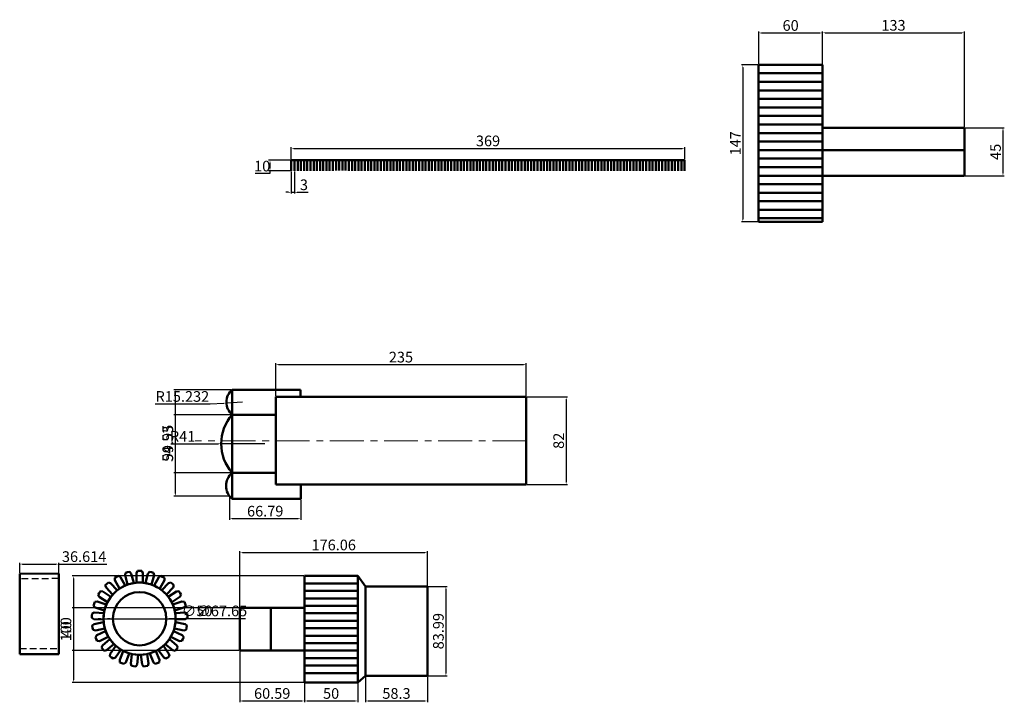
# Model space of a CAD drawing. Units: millimetres. Extents: x 828 to 2987, y 979 to 1807.
# Tile 6 of 6: x 2063 to 2987, y 979 to 1619. Entities that reach past the tile are written whole.
import ezdxf

# ---------------------------------------------------------------- set-up
doc = ezdxf.new("R2010")
doc.units = ezdxf.units.MM
doc.linetypes.add('CENTER', pattern=[50.8, 31.75, -6.35, 6.35, -6.35])
doc.linetypes.add('HIDDEN', pattern=[9.525, 6.35, -3.175])
for name, color, linetype, lineweight in [('M-CNTR', 1, 'CENTER', 18), ('M-DIMS', 2, 'Continuous', 25), ('M-HIDN', 4, 'HIDDEN', 25), ('M-OUTL', 7, 'Continuous', 50)]:
    doc.layers.add(name, color=color, linetype=linetype, lineweight=lineweight)
doc.styles.get("Standard").update_dxf_attribs({"font": 'arial.ttf'})
doc.dimstyles.new('ISO-25', dxfattribs={"dimtxt": 10, "dimasz": 2.5, "dimexe": 1.25, "dimexo": 0.625, "dimtad": 1, "dimtoh": 1, "dimdec": 0, "dimtxsty": 'Standard', "dimcen": 2.5, "dimadec": 0, "dimazin": 0, "dimtfac": 1, "dimtdec": 0, "dimtmove": 0, "dimatfit": 3, "dimfxl": 1, "dimarcsym": 0})

# ---------------------------------------------------------------- blocks, each defined once
blk = doc.blocks.new('*U61')
for p, q in [((-2, 5.46), (-3, 3.44)), ((-3, -5.56), (-3, 3.44)), ((0, 5.56), (-2, 5.46)), ((0, 5.56), (2, 5.46)), ((2, 5.46), (3, 3.44)), ((3, -5.56), (3, 3.44)), ((0, -5.56), (-3, -5.56)), ((0, -5.56), (3, -5.56))]:
    blk.add_line(p, q)
blk = doc.blocks.new('*U62')
at = {"layer": 'M-OUTL', "color": 0, "linetype": 'ByBlock', "lineweight": -2, "transparency": 16777216}
for p, rotation in [((2165.96, 1095.24), 14.39999999999996), ((2185.55, 1095.24), 345.6), ((2148.79, 1085.8), 43.20000000000002), ((2156.78, 1091.6), 28.79999999999999), ((2194.73, 1091.6), 331.2), ((2202.71, 1085.8), 316.8), ((2142.5, 1078.2), 57.6), ((2209.01, 1078.2), 302.4000000000001), ((2138.3, 1069.26), 72), ((2213.21, 1069.26), 288), ((2136.45, 1059.57), 86.40000000000002), ((2215.06, 1059.57), 273.6), ((2137.07, 1049.71), 100.8), ((2214.44, 1049.71), 259.2), ((2140.12, 1040.32), 115.2), ((2211.39, 1040.32), 244.7999999999999), ((2145.41, 1031.99), 129.6), ((2206.1, 1031.99), 230.4), ((2152.6, 1025.23), 144), ((2161.25, 1020.47), 158.4), ((2190.25, 1020.47), 201.6), ((2198.9, 1025.23), 216), ((2170.82, 1018.02), 172.8000000000001), ((2180.69, 1018.02), 187.1999999999999)]:
    blk.add_blockref('*U61', p, dxfattribs=dict(at, rotation=rotation))
blk.add_blockref('*U61', (2175.75, 1096.48), dxfattribs=at)
blk = doc.blocks.new('*D63')
at = {"layer": 'Defpoints', "color": 0, "transparency": 16777216}
for p in [(2538.55, 1265.06), (2538.55, 1182.82), (2576.02, 1182.82)]:
    blk.add_point(p, dxfattribs=at)
at = {"layer": 'M-DIMS', "color": 0, "lineweight": -2, "transparency": 16777216}
for p, q in [((2539.18, 1265.06), (2577.27, 1265.06)), ((2576.02, 1262.56), (2576.02, 1185.32)), ((2539.18, 1182.82), (2577.27, 1182.82))]:
    blk.add_line(p, q, dxfattribs=at)
at = {"layer": 'M-DIMS', "color": 0, "transparency": 16777216}
for points in [[(2575.61, 1262.56), (2576.44, 1262.56), (2576.02, 1265.06)], [(2575.61, 1185.32), (2576.44, 1185.32), (2576.02, 1182.82)]]:
    blk.add_solid(points, dxfattribs=at)
at = {"layer": 'M-DIMS', "color": 0, "transparency": 16777216, "insert": (2570.29, 1223.94), "char_height": 10, "attachment_point": 5, "rotation": 90}
blk.add_mtext('82', dxfattribs=at)
blk = doc.blocks.new('*D64')
at = {"layer": 'Defpoints', "color": 0, "transparency": 16777216}
for p in [(2538.55, 1295.39), (2303.51, 1265.06), (2538.55, 1265.06)]:
    blk.add_point(p, dxfattribs=at)
at = {"layer": 'M-DIMS', "color": 0, "lineweight": -2, "transparency": 16777216}
for p, q in [((2303.51, 1265.68), (2303.51, 1296.64)), ((2306.01, 1295.39), (2536.05, 1295.39)), ((2538.55, 1265.68), (2538.55, 1296.64))]:
    blk.add_line(p, q, dxfattribs=at)
at = {"layer": 'M-DIMS', "color": 0, "transparency": 16777216}
for points in [[(2306.01, 1295.8), (2306.01, 1294.97), (2303.51, 1295.39)], [(2536.05, 1295.8), (2536.05, 1294.97), (2538.55, 1295.39)]]:
    blk.add_solid(points, dxfattribs=at)
at = {"layer": 'M-DIMS', "color": 0, "transparency": 16777216, "insert": (2421.03, 1301.12), "char_height": 10, "attachment_point": 5}
blk.add_mtext('235', dxfattribs=at)
blk = doc.blocks.new('*D65')
at = {"layer": 'Defpoints', "color": 0, "transparency": 16777216}
for p in [(2687.32, 1498.16), (2318.12, 1487.03), (2687.32, 1487.03)]:
    blk.add_point(p, dxfattribs=at)
at = {"layer": 'M-DIMS', "color": 0, "lineweight": -2, "transparency": 16777216}
for p, q in [((2318.12, 1487.66), (2318.12, 1499.41)), ((2320.62, 1498.16), (2684.82, 1498.16)), ((2687.32, 1487.66), (2687.32, 1499.41))]:
    blk.add_line(p, q, dxfattribs=at)
at = {"layer": 'M-DIMS', "color": 0, "transparency": 16777216}
for points in [[(2320.62, 1498.57), (2320.62, 1497.74), (2318.12, 1498.16)], [(2684.82, 1498.57), (2684.82, 1497.74), (2687.32, 1498.16)]]:
    blk.add_solid(points, dxfattribs=at)
at = {"layer": 'M-DIMS', "color": 0, "transparency": 16777216, "insert": (2502.72, 1503.89), "char_height": 10, "attachment_point": 5}
blk.add_mtext('369', dxfattribs=at)
blk = doc.blocks.new('*D66')
at = {"layer": 'Defpoints', "color": 0, "transparency": 16777216}
for p in [(2816.67, 1606.42), (2756.67, 1576.58), (2816.67, 1576.58)]:
    blk.add_point(p, dxfattribs=at)
at = {"layer": 'M-DIMS', "color": 0, "lineweight": -2, "transparency": 16777216}
for p, q in [((2756.67, 1577.2), (2756.67, 1607.67)), ((2816.67, 1577.2), (2816.67, 1607.67)), ((2759.17, 1606.42), (2814.17, 1606.42))]:
    blk.add_line(p, q, dxfattribs=at)
at = {"layer": 'M-DIMS', "color": 0, "transparency": 16777216}
for points in [[(2759.17, 1606.84), (2759.17, 1606.01), (2756.67, 1606.42)], [(2814.17, 1606.84), (2814.17, 1606.01), (2816.67, 1606.42)]]:
    blk.add_solid(points, dxfattribs=at)
at = {"layer": 'M-DIMS', "color": 0, "transparency": 16777216, "insert": (2786.67, 1612.15), "char_height": 10, "attachment_point": 5}
blk.add_mtext('60', dxfattribs=at)
blk = doc.blocks.new('*D67')
at = {"layer": 'Defpoints', "color": 0, "transparency": 16777216}
for p in [(2756.67, 1576.58), (2741.8, 1429.28), (2756.67, 1429.28)]:
    blk.add_point(p, dxfattribs=at)
at = {"layer": 'M-DIMS', "color": 0, "lineweight": -2, "transparency": 16777216}
for p, q in [((2756.04, 1576.58), (2740.55, 1576.58)), ((2741.8, 1574.08), (2741.8, 1431.78)), ((2756.04, 1429.28), (2740.55, 1429.28))]:
    blk.add_line(p, q, dxfattribs=at)
at = {"layer": 'M-DIMS', "color": 0, "transparency": 16777216}
for points in [[(2741.38, 1574.08), (2742.21, 1574.08), (2741.8, 1576.58)], [(2741.38, 1431.78), (2742.21, 1431.78), (2741.8, 1429.28)]]:
    blk.add_solid(points, dxfattribs=at)
at = {"layer": 'M-DIMS', "color": 0, "transparency": 16777216, "insert": (2736.15, 1502.93), "char_height": 10, "attachment_point": 5, "rotation": 90}
blk.add_mtext('147', dxfattribs=at)
blk = doc.blocks.new('*D68')
at = {"layer": 'Defpoints', "color": 0, "transparency": 16777216}
for p in [(2949.69, 1606.56), (2816.67, 1517.31), (2949.69, 1517.31)]:
    blk.add_point(p, dxfattribs=at)
at = {"layer": 'M-DIMS', "color": 0, "lineweight": -2, "transparency": 16777216}
for p, q in [((2816.67, 1517.93), (2816.67, 1607.81)), ((2949.69, 1517.93), (2949.69, 1607.81)), ((2819.17, 1606.56), (2947.19, 1606.56))]:
    blk.add_line(p, q, dxfattribs=at)
at = {"layer": 'M-DIMS', "color": 0, "transparency": 16777216}
for points in [[(2819.17, 1606.98), (2819.17, 1606.14), (2816.67, 1606.56)], [(2947.19, 1606.98), (2947.19, 1606.14), (2949.69, 1606.56)]]:
    blk.add_solid(points, dxfattribs=at)
at = {"layer": 'M-DIMS', "color": 0, "transparency": 16777216, "insert": (2883.18, 1612.29), "char_height": 10, "attachment_point": 5}
blk.add_mtext('133', dxfattribs=at)
blk = doc.blocks.new('*D69')
at = {"layer": 'Defpoints', "color": 0, "transparency": 16777216}
for p in [(2949.69, 1517.31), (2949.69, 1472.54), (2985.91, 1472.54)]:
    blk.add_point(p, dxfattribs=at)
at = {"layer": 'M-DIMS', "color": 0, "lineweight": -2, "transparency": 16777216}
for p, q in [((2950.32, 1517.31), (2987.16, 1517.31)), ((2985.91, 1514.81), (2985.91, 1475.04)), ((2950.32, 1472.54), (2987.16, 1472.54))]:
    blk.add_line(p, q, dxfattribs=at)
at = {"layer": 'M-DIMS', "color": 0, "transparency": 16777216}
for points in [[(2985.49, 1514.81), (2986.33, 1514.81), (2985.91, 1517.31)], [(2985.49, 1475.04), (2986.33, 1475.04), (2985.91, 1472.54)]]:
    blk.add_solid(points, dxfattribs=at)
at = {"layer": 'M-DIMS', "color": 0, "transparency": 16777216, "insert": (2980.2, 1494.92), "char_height": 10, "attachment_point": 5, "rotation": 90}
blk.add_mtext('45', dxfattribs=at)
blk = doc.blocks.new('*D99')
at = {"layer": 'Defpoints', "color": 0, "transparency": 16777216}
for p in [(2318.12, 1487.03), (2298.12, 1477.03), (2318.12, 1477.03)]:
    blk.add_point(p, dxfattribs=at)
at = {"layer": 'M-DIMS', "color": 0, "lineweight": -2, "transparency": 16777216}
for p, q in [((2317.49, 1487.03), (2296.87, 1487.03)), ((2298.12, 1484.53), (2298.12, 1479.53)), ((2298.12, 1474.53), (2284.14, 1474.53)), ((2317.49, 1477.03), (2296.87, 1477.03)), ((2298.12, 1477.03), (2298.12, 1474.53))]:
    blk.add_line(p, q, dxfattribs=at)
at = {"layer": 'M-DIMS', "color": 0, "transparency": 16777216}
for points in [[(2297.7, 1484.53), (2298.53, 1484.53), (2298.12, 1487.03)], [(2297.7, 1479.53), (2298.53, 1479.53), (2298.12, 1477.03)]]:
    blk.add_solid(points, dxfattribs=at)
at = {"layer": 'M-DIMS', "color": 0, "transparency": 16777216, "insert": (2290.82, 1480.26), "char_height": 10, "attachment_point": 5}
blk.add_mtext('10', dxfattribs=at)
blk = doc.blocks.new('*D100')
at = {"layer": 'Defpoints', "color": 0, "transparency": 16777216}
for p in [(2318.12, 1477.03), (2321.12, 1477.03), (2321.12, 1456.98)]:
    blk.add_point(p, dxfattribs=at)
at = {"layer": 'M-DIMS', "color": 0, "lineweight": -2, "transparency": 16777216}
for p, q in [((2318.12, 1476.41), (2318.12, 1455.73)), ((2321.12, 1476.41), (2321.12, 1455.73)), ((2315.62, 1456.98), (2313.12, 1456.98)), ((2318.12, 1456.98), (2321.12, 1456.98)), ((2323.62, 1456.98), (2333.91, 1456.98))]:
    blk.add_line(p, q, dxfattribs=at)
at = {"layer": 'M-DIMS', "color": 0, "transparency": 16777216}
for points in [[(2315.62, 1457.4), (2315.62, 1456.57), (2318.12, 1456.98)], [(2323.62, 1457.4), (2323.62, 1456.57), (2321.12, 1456.98)]]:
    blk.add_solid(points, dxfattribs=at)
at = {"layer": 'M-DIMS', "color": 0, "transparency": 16777216, "insert": (2330.01, 1462.72), "char_height": 10, "attachment_point": 5}
blk.add_mtext('3', dxfattribs=at)
blk = doc.blocks.new('*D101')
at = {"layer": 'Defpoints', "color": 0, "transparency": 16777216}
for p in [(2262.71, 1271.88), (2209.27, 1171.93), (2260.25, 1171.93)]:
    blk.add_point(p, dxfattribs=at)
at = {"layer": 'M-DIMS', "color": 0, "lineweight": -2, "transparency": 16777216}
for p, q in [((2262.09, 1271.88), (2208.02, 1271.88)), ((2209.27, 1269.38), (2209.27, 1174.43)), ((2259.62, 1171.93), (2208.02, 1171.93))]:
    blk.add_line(p, q, dxfattribs=at)
at = {"layer": 'M-DIMS', "color": 0, "transparency": 16777216}
for points in [[(2208.85, 1269.38), (2209.68, 1269.38), (2209.27, 1271.88)], [(2208.85, 1174.43), (2209.68, 1174.43), (2209.27, 1171.93)]]:
    blk.add_solid(points, dxfattribs=at)
at = {"layer": 'M-DIMS', "color": 0, "transparency": 16777216, "insert": (2203.54, 1221.9), "char_height": 10, "attachment_point": 5, "rotation": 90}
blk.add_mtext('99.95', dxfattribs=at)
blk = doc.blocks.new('*D102')
at = {"layer": 'Defpoints', "color": 0, "transparency": 16777216}
for p in [(2262.71, 1248.42), (2209.27, 1193.89), (2262.71, 1193.89)]:
    blk.add_point(p, dxfattribs=at)
at = {"layer": 'M-DIMS', "color": 0, "lineweight": -2, "transparency": 16777216}
for p, q in [((2262.09, 1248.42), (2208.02, 1248.42)), ((2209.27, 1245.92), (2209.27, 1196.39)), ((2262.09, 1193.89), (2208.02, 1193.89))]:
    blk.add_line(p, q, dxfattribs=at)
at = {"layer": 'M-DIMS', "color": 0, "transparency": 16777216}
for points in [[(2208.85, 1245.92), (2209.68, 1245.92), (2209.27, 1248.42)], [(2208.85, 1196.39), (2209.68, 1196.39), (2209.27, 1193.89)]]:
    blk.add_solid(points, dxfattribs=at)
at = {"layer": 'M-DIMS', "color": 0, "transparency": 16777216, "insert": (2203.53, 1221.16), "char_height": 10, "attachment_point": 5, "rotation": 90}
blk.add_mtext('54.53', dxfattribs=at)
blk = doc.blocks.new('*D103')
at = {"layer": 'Defpoints', "color": 0, "transparency": 16777216}
for p in [(2260.25, 1171.93), (2327.04, 1169.42), (2327.04, 1150.92)]:
    blk.add_point(p, dxfattribs=at)
at = {"layer": 'M-DIMS', "color": 0, "lineweight": -2, "transparency": 16777216}
for p, q in [((2260.25, 1171.31), (2260.25, 1149.67)), ((2327.04, 1168.8), (2327.04, 1149.67)), ((2262.75, 1150.92), (2324.54, 1150.92))]:
    blk.add_line(p, q, dxfattribs=at)
at = {"layer": 'M-DIMS', "color": 0, "transparency": 16777216}
for points in [[(2262.75, 1151.34), (2262.75, 1150.51), (2260.25, 1150.92)], [(2324.54, 1151.34), (2324.54, 1150.51), (2327.04, 1150.92)]]:
    blk.add_solid(points, dxfattribs=at)
at = {"layer": 'M-DIMS', "color": 0, "transparency": 16777216, "insert": (2293.64, 1156.65), "char_height": 10, "attachment_point": 5}
blk.add_mtext('66.79', dxfattribs=at)
blk = doc.blocks.new('*D104')
at = {"layer": 'Defpoints', "color": 0, "transparency": 16777216}
for p in [(2099.87, 1108.29), (2063.26, 1099.09), (2099.87, 1099.39)]:
    blk.add_point(p, dxfattribs=at)
at = {"layer": 'M-DIMS', "color": 0, "lineweight": -2, "transparency": 16777216}
for p, q in [((2063.26, 1099.71), (2063.26, 1109.54)), ((2099.87, 1100.01), (2099.87, 1109.54)), ((2065.76, 1108.29), (2097.37, 1108.29)), ((2099.87, 1108.29), (2145.09, 1108.29))]:
    blk.add_line(p, q, dxfattribs=at)
at = {"layer": 'M-DIMS', "color": 0, "transparency": 16777216}
for points in [[(2065.76, 1108.7), (2065.76, 1107.87), (2063.26, 1108.29)], [(2097.37, 1108.7), (2097.37, 1107.87), (2099.87, 1108.29)]]:
    blk.add_solid(points, dxfattribs=at)
at = {"layer": 'M-DIMS', "color": 0, "transparency": 16777216, "insert": (2123.73, 1114.02), "char_height": 10, "attachment_point": 5}
blk.add_mtext('36.614', dxfattribs=at)
blk = doc.blocks.new('*D105')
at = {"layer": 'Defpoints', "color": 0, "transparency": 16777216}
for p in [(2269.9, 1027.14), (2330.49, 1027.14), (2330.49, 979.94)]:
    blk.add_point(p, dxfattribs=at)
at = {"layer": 'M-DIMS', "color": 0, "lineweight": -2, "transparency": 16777216}
for p, q in [((2269.9, 1026.51), (2269.9, 978.69)), ((2330.49, 1026.51), (2330.49, 978.69)), ((2272.4, 979.94), (2327.99, 979.94))]:
    blk.add_line(p, q, dxfattribs=at)
at = {"layer": 'M-DIMS', "color": 0, "transparency": 16777216}
for points in [[(2272.4, 980.36), (2272.4, 979.52), (2269.9, 979.94)], [(2327.99, 980.36), (2327.99, 979.52), (2330.49, 979.94)]]:
    blk.add_solid(points, dxfattribs=at)
at = {"layer": 'M-DIMS', "color": 0, "transparency": 16777216, "insert": (2300.19, 985.67), "char_height": 10, "attachment_point": 5}
blk.add_mtext('60.59', dxfattribs=at)
blk = doc.blocks.new('*D106')
at = {"layer": 'Defpoints', "color": 0, "transparency": 16777216}
for p in [(2330.49, 997.14), (2380.49, 997.14), (2380.49, 979.94)]:
    blk.add_point(p, dxfattribs=at)
at = {"layer": 'M-DIMS', "color": 0, "lineweight": -2, "transparency": 16777216}
for p, q in [((2330.49, 996.51), (2330.49, 978.69)), ((2380.49, 996.51), (2380.49, 978.69)), ((2332.99, 979.94), (2377.99, 979.94))]:
    blk.add_line(p, q, dxfattribs=at)
at = {"layer": 'M-DIMS', "color": 0, "transparency": 16777216}
for points in [[(2332.99, 980.36), (2332.99, 979.52), (2330.49, 979.94)], [(2377.99, 980.36), (2377.99, 979.52), (2380.49, 979.94)]]:
    blk.add_solid(points, dxfattribs=at)
at = {"layer": 'M-DIMS', "color": 0, "transparency": 16777216, "insert": (2355.49, 985.67), "char_height": 10, "attachment_point": 5}
blk.add_mtext('50', dxfattribs=at)
blk = doc.blocks.new('*D107')
at = {"layer": 'Defpoints', "color": 0, "transparency": 16777216}
for p in [(2387.67, 1003.41), (2445.96, 1003.41), (2445.96, 979.94)]:
    blk.add_point(p, dxfattribs=at)
at = {"layer": 'M-DIMS', "color": 0, "lineweight": -2, "transparency": 16777216}
for p, q in [((2387.67, 1002.78), (2387.67, 978.69)), ((2445.96, 1002.78), (2445.96, 978.69)), ((2390.17, 979.94), (2443.46, 979.94))]:
    blk.add_line(p, q, dxfattribs=at)
at = {"layer": 'M-DIMS', "color": 0, "transparency": 16777216}
for points in [[(2390.17, 980.36), (2390.17, 979.52), (2387.67, 979.94)], [(2443.46, 980.36), (2443.46, 979.52), (2445.96, 979.94)]]:
    blk.add_solid(points, dxfattribs=at)
at = {"layer": 'M-DIMS', "color": 0, "transparency": 16777216, "insert": (2416.82, 985.67), "char_height": 10, "attachment_point": 5}
blk.add_mtext('58.3', dxfattribs=at)
blk = doc.blocks.new('*D108')
at = {"layer": 'Defpoints', "color": 0, "transparency": 16777216}
for p in [(2445.96, 1119.23), (2269.9, 1027.14), (2445.96, 1003.41)]:
    blk.add_point(p, dxfattribs=at)
at = {"layer": 'M-DIMS', "color": 0, "lineweight": -2, "transparency": 16777216}
for p, q in [((2269.9, 1027.76), (2269.9, 1120.48)), ((2272.4, 1119.23), (2443.46, 1119.23)), ((2445.96, 1004.03), (2445.96, 1120.48))]:
    blk.add_line(p, q, dxfattribs=at)
at = {"layer": 'M-DIMS', "color": 0, "transparency": 16777216}
for points in [[(2272.4, 1119.65), (2272.4, 1118.82), (2269.9, 1119.23)], [(2443.46, 1119.65), (2443.46, 1118.82), (2445.96, 1119.23)]]:
    blk.add_solid(points, dxfattribs=at)
at = {"layer": 'M-DIMS', "color": 0, "transparency": 16777216, "insert": (2357.93, 1124.96), "char_height": 10, "attachment_point": 5}
blk.add_mtext('176.06', dxfattribs=at)
blk = doc.blocks.new('*D109')
at = {"layer": 'Defpoints', "color": 0, "transparency": 16777216}
for p in [(2269.9, 1067.14), (2113.67, 1027.14), (2269.9, 1027.14)]:
    blk.add_point(p, dxfattribs=at)
at = {"layer": 'M-DIMS', "color": 0, "lineweight": -2, "transparency": 16777216}
for p, q in [((2269.28, 1067.14), (2112.42, 1067.14)), ((2113.67, 1064.64), (2113.67, 1029.64)), ((2269.28, 1027.14), (2112.42, 1027.14))]:
    blk.add_line(p, q, dxfattribs=at)
at = {"layer": 'M-DIMS', "color": 0, "transparency": 16777216}
for points in [[(2113.25, 1064.64), (2114.09, 1064.64), (2113.67, 1067.14)], [(2113.25, 1029.64), (2114.09, 1029.64), (2113.67, 1027.14)]]:
    blk.add_solid(points, dxfattribs=at)
at = {"layer": 'M-DIMS', "color": 0, "transparency": 16777216, "insert": (2107.94, 1047.14), "char_height": 10, "attachment_point": 5, "rotation": 90}
blk.add_mtext('40', dxfattribs=at)
blk = doc.blocks.new('*D110')
at = {"layer": 'Defpoints', "color": 0, "transparency": 16777216}
for p in [(2330.49, 1097.14), (2113.67, 997.14), (2330.49, 997.14)]:
    blk.add_point(p, dxfattribs=at)
at = {"layer": 'M-DIMS', "color": 0, "lineweight": -2, "transparency": 16777216}
for p, q in [((2329.86, 1097.14), (2112.42, 1097.14)), ((2113.67, 1094.64), (2113.67, 999.64)), ((2329.86, 997.14), (2112.42, 997.14))]:
    blk.add_line(p, q, dxfattribs=at)
at = {"layer": 'M-DIMS', "color": 0, "transparency": 16777216}
for points in [[(2113.25, 1094.64), (2114.09, 1094.64), (2113.67, 1097.14)], [(2113.25, 999.64), (2114.09, 999.64), (2113.67, 997.14)]]:
    blk.add_solid(points, dxfattribs=at)
at = {"layer": 'M-DIMS', "color": 0, "transparency": 16777216, "insert": (2107.94, 1047.14), "char_height": 10, "attachment_point": 5, "rotation": 90}
blk.add_mtext('100', dxfattribs=at)
blk = doc.blocks.new('*D111')
at = {"layer": 'Defpoints', "color": 0, "transparency": 16777216}
for p in [(2445.96, 1087.4), (2445.96, 1003.41), (2463.16, 1003.41)]:
    blk.add_point(p, dxfattribs=at)
at = {"layer": 'M-DIMS', "color": 0, "lineweight": -2, "transparency": 16777216}
for p, q in [((2446.59, 1087.4), (2464.41, 1087.4)), ((2463.16, 1084.9), (2463.16, 1005.91)), ((2446.59, 1003.41), (2464.41, 1003.41))]:
    blk.add_line(p, q, dxfattribs=at)
at = {"layer": 'M-DIMS', "color": 0, "transparency": 16777216}
for points in [[(2462.75, 1084.9), (2463.58, 1084.9), (2463.16, 1087.4)], [(2462.75, 1005.91), (2463.58, 1005.91), (2463.16, 1003.41)]]:
    blk.add_solid(points, dxfattribs=at)
at = {"layer": 'M-DIMS', "color": 0, "transparency": 16777216, "insert": (2457.43, 1045.4), "char_height": 10, "attachment_point": 5, "rotation": 90}
blk.add_mtext('83.99', dxfattribs=at)
blk = doc.blocks.new('*D141')
at = {"layer": 'Defpoints', "color": 0, "transparency": 16777216}
for p in [(2252.33, 1221.16), (2293.33, 1221.16)]:
    blk.add_point(p, dxfattribs=at)
at = {"layer": 'M-DIMS', "color": 0, "lineweight": -2, "transparency": 16777216}
for p, q in [((2205.14, 1221.16), (2227.73, 1221.16)), ((2227.73, 1221.16), (2249.83, 1221.16)), ((2293.33, 1221.16), (2252.33, 1221.16))]:
    blk.add_line(p, q, dxfattribs=at)
at = {"layer": 'M-DIMS', "color": 0, "transparency": 16777216}
blk.add_solid([(2249.83, 1221.57), (2249.83, 1220.74), (2252.33, 1221.16)], dxfattribs=at)
at = {"layer": 'M-DIMS', "color": 0, "transparency": 16777216, "insert": (2216.13, 1226.8), "char_height": 10, "attachment_point": 5}
blk.add_mtext('R41', dxfattribs=at)
blk = doc.blocks.new('*D142')
at = {"layer": 'Defpoints', "color": 0, "transparency": 16777216}
for p in [(2257.22, 1259.32), (2272.43, 1260.15)]:
    blk.add_point(p, dxfattribs=at)
at = {"layer": 'M-DIMS', "color": 0, "lineweight": -2, "transparency": 16777216}
for p, q in [((2190.42, 1258.49), (2242.02, 1258.49)), ((2242.02, 1258.49), (2254.72, 1259.18)), ((2272.43, 1260.15), (2257.22, 1259.32))]:
    blk.add_line(p, q, dxfattribs=at)
at = {"layer": 'M-DIMS', "color": 0, "transparency": 16777216}
blk.add_solid([(2254.7, 1259.6), (2254.75, 1258.77), (2257.22, 1259.32)], dxfattribs=at)
at = {"layer": 'M-DIMS', "color": 0, "transparency": 16777216, "insert": (2215.91, 1264.22), "char_height": 10, "attachment_point": 5}
blk.add_mtext('R15.232', dxfattribs=at)
blk = doc.blocks.new('*D143')
at = {"layer": 'Defpoints', "color": 0, "transparency": 16777216}
for p in [(2150.75, 1057.09), (2200.75, 1057.09)]:
    blk.add_point(p, dxfattribs=at)
at = {"layer": 'M-DIMS', "color": 0, "lineweight": -2, "transparency": 16777216}
for p, q in [((2148.25, 1057.09), (2145.75, 1057.09)), ((2150.75, 1057.09), (2200.75, 1057.09)), ((2216.52, 1057.09), (2203.25, 1057.09)), ((2242.32, 1057.09), (2216.52, 1057.09))]:
    blk.add_line(p, q, dxfattribs=at)
at = {"layer": 'M-DIMS', "color": 0, "transparency": 16777216}
for points in [[(2148.25, 1057.51), (2148.25, 1056.68), (2150.75, 1057.09)], [(2203.25, 1057.51), (2203.25, 1056.68), (2200.75, 1057.09)]]:
    blk.add_solid(points, dxfattribs=at)
at = {"layer": 'M-DIMS', "color": 0, "transparency": 16777216, "insert": (2229.73, 1063.1), "char_height": 10, "attachment_point": 5}
blk.add_mtext('∅50', dxfattribs=at)
blk = doc.blocks.new('*D144')
at = {"layer": 'Defpoints', "color": 0, "transparency": 16777216}
for p in [(2141.93, 1057.09), (2209.58, 1057.09)]:
    blk.add_point(p, dxfattribs=at)
at = {"layer": 'M-DIMS', "color": 0, "lineweight": -2, "transparency": 16777216}
for p, q in [((2139.43, 1057.09), (2136.93, 1057.09)), ((2141.93, 1057.09), (2209.58, 1057.09)), ((2229.88, 1057.09), (2212.08, 1057.09)), ((2275.2, 1057.09), (2229.88, 1057.09))]:
    blk.add_line(p, q, dxfattribs=at)
at = {"layer": 'M-DIMS', "color": 0, "transparency": 16777216}
for points in [[(2139.43, 1057.51), (2139.43, 1056.68), (2141.93, 1057.09)], [(2212.08, 1057.51), (2212.08, 1056.68), (2209.58, 1057.09)]]:
    blk.add_solid(points, dxfattribs=at)
at = {"layer": 'M-DIMS', "color": 0, "transparency": 16777216, "insert": (2252.85, 1063.1), "char_height": 10, "attachment_point": 5}
blk.add_mtext('∅67.65', dxfattribs=at)

msp = doc.modelspace()

# ---------------------------------------------------------------- linework, layer by layer
at = {"layer": 'M-CNTR'}
msp.add_line((2538.5542, 1223.9389), (2227.7676, 1223.9389), dxfattribs=at)
at = {"layer": 'M-HIDN'}
for p, q in [((2099.9133, 1094.7014), (2063.2995, 1094.4015)), ((2063.2612, 1029.0021), (2099.8749, 1029.0021))]:
    msp.add_line(p, q, dxfattribs=at)
at = {"layer": 'M-OUTL'}
for p, q in [((2756.6676, 1576.5779), (2756.6676, 1429.2768)), ((2756.6676, 1576.5779), (2816.6676, 1576.5779)), ((2756.6676, 1576.5779), (2756.6676, 1568.5779)), ((2816.6676, 1429.2768), (2816.6676, 1576.5779)), ((2756.6676, 1568.5779), (2816.6676, 1568.5779)), ((2816.6676, 1560.5779), (2756.6676, 1560.5779)), ((2756.6676, 1552.5779), (2816.6676, 1552.5779)), ((2816.6676, 1544.5779), (2756.6676, 1544.5779)), ((2756.6676, 1536.5779), (2816.6676, 1536.5779)), ((2816.6676, 1528.5779), (2756.6676, 1528.5779)), ((2756.6676, 1520.5779), (2816.6676, 1520.5779)), ((2816.6676, 1517.308), (2949.693, 1517.308)), ((2949.693, 1517.308), (2949.693, 1472.5387)), ((2816.6676, 1512.5779), (2756.6676, 1512.5779)), ((2756.6676, 1504.5779), (2816.6676, 1504.5779)), ((2816.6676, 1496.5779), (2756.6676, 1496.5779)), ((2756.6676, 1488.5779), (2816.6676, 1488.5779)), ((2816.6676, 1496.5779), (2949.693, 1496.5779)), ((2318.1154, 1487.0339), (2687.1154, 1487.0339)), ((2318.1154, 1487.0339), (2318.1154, 1477.0339)), ((2321.1154, 1477.0339), (2321.1154, 1487.0339)), ((2321.1154, 1487.0339), (2324.1154, 1487.0339)), ((2324.1154, 1487.0339), (2324.1154, 1477.0339)), ((2327.1154, 1477.0339), (2327.1154, 1487.0339)), ((2330.1154, 1487.0339), (2330.1154, 1476.9825)), ((2333.1154, 1476.9825), (2333.1154, 1487.0339)), ((2336.1154, 1487.0339), (2336.1154, 1477.0762)), ((2339.1154, 1477.0762), (2339.1154, 1487.0339)), ((2342.1154, 1487.0339), (2342.1154, 1477.0339)), ((2345.1154, 1477.0339), (2345.1154, 1487.0339)), ((2348.1154, 1487.0339), (2348.1154, 1477.1476)), ((2351.1154, 1477.1476), (2351.1154, 1487.0339)), ((2354.1154, 1487.0339), (2354.1154, 1477.1238)), ((2357.1154, 1477.1238), (2357.1154, 1487.0339)), ((2360.1154, 1487.0339), (2360.1154, 1477.4097)), ((2363.1154, 1477.4097), (2363.1154, 1487.0339)), ((2366.1154, 1487.0339), (2366.1154, 1477.2911)), ((2369.1154, 1477.2911), (2369.1154, 1487.0339)), ((2372.1154, 1487.0339), (2372.1154, 1477.1482)), ((2375.1154, 1477.1482), (2375.1154, 1487.0339)), ((2378.1154, 1487.0339), (2378.1154, 1477.0474)), ((2381.1154, 1477.0474), (2381.1154, 1487.0339)), ((2384.1154, 1487.0339), (2384.1154, 1477.0857)), ((2387.1154, 1477.0857), (2387.1154, 1487.0339)), ((2390.1154, 1487.0339), (2390.1154, 1477.0339)), ((2393.1154, 1477.0339), (2393.1154, 1487.0339)), ((2396.1154, 1487.0339), (2396.1154, 1477.0339)), ((2399.1154, 1477.0339), (2399.1154, 1487.0339)), ((2402.1154, 1487.0339), (2402.1154, 1477.0339)), ((2405.1154, 1477.0339), (2405.1154, 1487.0339)), ((2408.1154, 1487.0339), (2408.1154, 1477.0339)), ((2411.1154, 1477.0339), (2411.1154, 1487.0339)), ((2414.1154, 1487.0339), (2414.1154, 1477.0339)), ((2417.1154, 1477.0339), (2417.1154, 1487.0339)), ((2420.1154, 1487.0339), (2420.1154, 1477.0339)), ((2423.1154, 1477.0339), (2423.1154, 1487.0339)), ((2426.1154, 1487.0339), (2426.1154, 1477.0339)), ((2429.1154, 1477.0339), (2429.1154, 1487.0339)), ((2432.1154, 1487.0339), (2432.1154, 1477.0339)), ((2435.1154, 1477.0339), (2435.1154, 1487.0339)), ((2438.1154, 1487.0339), (2438.1154, 1477.0339)), ((2441.1154, 1477.0339), (2441.1154, 1487.0339)), ((2444.1154, 1487.0339), (2444.1154, 1477.0339)), ((2447.1154, 1477.0339), (2447.1154, 1487.0339)), ((2450.1154, 1487.0339), (2450.1154, 1477.0339)), ((2453.1154, 1477.0339), (2453.1154, 1487.0339)), ((2456.1154, 1487.0339), (2456.1154, 1477.0339)), ((2459.1154, 1477.0339), (2459.1154, 1487.0339)), ((2462.1154, 1487.0339), (2462.1154, 1477.0339)), ((2465.1154, 1477.0339), (2465.1154, 1487.0339)), ((2468.1154, 1487.0339), (2468.1154, 1477.0339)), ((2471.1154, 1477.0339), (2471.1154, 1487.0339)), ((2474.1154, 1487.0339), (2474.1154, 1477.0339)), ((2477.1154, 1477.0339), (2477.1154, 1487.0339)), ((2480.1154, 1487.0339), (2480.1154, 1477.0339)), ((2483.1154, 1477.0339), (2483.1154, 1487.0339)), ((2486.1154, 1487.0339), (2486.1154, 1477.0339)), ((2489.1154, 1477.0339), (2489.1154, 1487.0339)), ((2492.1154, 1487.0339), (2492.1154, 1477.0339)), ((2495.1154, 1477.0339), (2495.1154, 1487.0339)), ((2498.1154, 1487.0339), (2498.1154, 1477.0339)), ((2501.1154, 1477.0339), (2501.1154, 1487.0339)), ((2504.1154, 1487.0339), (2504.1154, 1477.0339)), ((2507.1154, 1477.0339), (2507.1154, 1487.0339)), ((2510.1154, 1487.0339), (2510.1154, 1477.0339)), ((2513.1154, 1477.0339), (2513.1154, 1487.0339)), ((2516.1154, 1487.0339), (2516.1154, 1477.0339)), ((2519.1154, 1477.0339), (2519.1154, 1487.0339)), ((2522.1154, 1487.0339), (2522.1154, 1477.0339)), ((2525.1154, 1477.0339), (2525.1154, 1487.0339)), ((2528.1154, 1487.0339), (2528.1154, 1477.0339)), ((2531.1154, 1477.0339), (2531.1154, 1487.0339)), ((2534.1154, 1487.0339), (2534.1154, 1477.0339)), ((2537.1154, 1477.0339), (2537.1154, 1487.0339)), ((2540.1154, 1487.0339), (2540.1154, 1477.0339)), ((2543.1154, 1477.0339), (2543.1154, 1487.0339)), ((2546.1154, 1487.0339), (2546.1154, 1477.0339)), ((2549.1154, 1477.0339), (2549.1154, 1487.0339)), ((2552.1154, 1487.0339), (2552.1154, 1477.0339)), ((2555.1154, 1477.0339), (2555.1154, 1487.0339)), ((2558.1154, 1487.0339), (2558.1154, 1477.0339)), ((2561.1154, 1477.0339), (2561.1154, 1487.0339)), ((2564.1154, 1487.0339), (2564.1154, 1477.0339)), ((2567.1154, 1477.0339), (2567.1154, 1487.0339)), ((2570.1154, 1487.0339), (2570.1154, 1477.0339)), ((2573.1154, 1477.0339), (2573.1154, 1487.0339)), ((2576.1154, 1487.0339), (2576.1154, 1477.0339)), ((2579.1154, 1477.0339), (2579.1154, 1487.0339)), ((2582.1154, 1487.0339), (2582.1154, 1477.0339)), ((2585.1154, 1477.0339), (2585.1154, 1487.0339)), ((2588.1154, 1487.0339), (2588.1154, 1477.0339)), ((2591.1154, 1477.0339), (2591.1154, 1487.0339)), ((2594.1154, 1487.0339), (2594.1154, 1477.0339)), ((2597.1154, 1477.0339), (2597.1154, 1487.0339)), ((2600.1154, 1487.0339), (2600.1154, 1477.0339)), ((2603.1154, 1477.0339), (2603.1154, 1487.0339)), ((2606.1154, 1487.0339), (2606.1154, 1477.0339)), ((2609.1154, 1477.0339), (2609.1154, 1487.0339)), ((2612.1154, 1487.0339), (2612.1154, 1477.0339)), ((2615.1154, 1477.0339), (2615.1154, 1487.0339)), ((2618.1154, 1487.0339), (2618.1154, 1477.0339)), ((2621.1154, 1477.0339), (2621.1154, 1487.0339)), ((2624.1154, 1487.0339), (2624.1154, 1477.0339)), ((2627.1154, 1477.0339), (2627.1154, 1487.0339)), ((2630.1154, 1487.0339), (2630.1154, 1477.0339)), ((2633.1154, 1477.0339), (2633.1154, 1487.0339)), ((2636.1154, 1487.0339), (2636.1154, 1477.0339)), ((2639.1154, 1477.0339), (2639.1154, 1487.0339)), ((2642.1154, 1487.0339), (2642.1154, 1477.0339)), ((2645.1154, 1477.0339), (2645.1154, 1487.0339)), ((2648.1154, 1487.0339), (2648.1154, 1477.0339)), ((2651.1154, 1477.0339), (2651.1154, 1487.0339)), ((2654.1154, 1487.0339), (2654.1154, 1477.0339)), ((2657.1154, 1477.0339), (2657.1154, 1487.0339)), ((2660.1154, 1487.0339), (2660.1154, 1477.0339)), ((2663.1154, 1477.0339), (2663.1154, 1487.0339)), ((2666.1154, 1487.0339), (2666.1154, 1477.0339)), ((2669.1154, 1477.0339), (2669.1154, 1487.0339)), ((2672.1154, 1487.0339), (2672.1154, 1477.0339)), ((2675.1154, 1477.0339), (2675.1154, 1487.0339)), ((2678.1154, 1487.0339), (2678.1154, 1477.0339)), ((2681.1154, 1477.0339), (2681.1154, 1487.0339)), ((2684.1154, 1487.0339), (2684.1154, 1477.0339)), ((2687.1154, 1485.3545), (2687.1154, 1487.0339)), ((2687.1154, 1477.0339), (2687.1154, 1485.3545)), ((2816.6676, 1480.5779), (2756.6676, 1480.5779)), ((2756.6676, 1472.5779), (2816.6676, 1472.5779)), ((2816.6676, 1472.5387), (2949.693, 1472.5387)), ((2816.6676, 1464.5779), (2756.6676, 1464.5779)), ((2756.6676, 1456.5779), (2816.6676, 1456.5779)), ((2816.6676, 1448.5779), (2756.6676, 1448.5779)), ((2756.6676, 1440.5779), (2816.6676, 1440.5779)), ((2816.6676, 1432.5779), (2756.6676, 1432.5779)), ((2756.6676, 1429.2768), (2816.6676, 1429.2768)), ((2262.7106, 1248.4192), (2262.7106, 1271.8788)), ((2262.7106, 1271.8788), (2326.8714, 1271.8788)), ((2326.8714, 1271.8788), (2326.8714, 1265.0585)), ((2303.5105, 1265.0585), (2538.5542, 1265.0585)), ((2303.5105, 1265.0585), (2303.5105, 1182.8194)), ((2538.5542, 1265.0585), (2538.5542, 1182.8194)), ((2262.7106, 1248.4192), (2303.5105, 1248.4192)), ((2262.7106, 1248.4192), (2262.7106, 1169.4235)), ((2303.5105, 1193.8924), (2262.7106, 1193.8924)), ((2538.5542, 1182.8194), (2303.5105, 1182.8194)), ((2327.0396, 1169.4235), (2327.0396, 1182.8194)), ((2262.7106, 1169.4235), (2327.0396, 1169.4235)), ((2099.8749, 1099.3864), (2063.2612, 1099.0866)), ((2063.2612, 1099.0866), (2063.2612, 1023.8241)), ((2099.8749, 1023.8241), (2099.8749, 1099.3864)), ((2330.4889, 1097.1395), (2330.4889, 997.1395)), ((2380.4889, 1097.1395), (2330.4889, 1097.1395)), ((2330.4889, 1097.1395), (2330.4889, 1094.1395)), ((2330.4889, 1097.1395), (2330.4889, 1090.1395)), ((2380.4889, 997.1395), (2380.4889, 1097.1395)), ((2380.4889, 1097.1395), (2387.6697, 1087.396)), ((2330.4889, 1090.1395), (2380.4889, 1090.1395)), ((2380.4889, 1083.1395), (2330.4889, 1083.1395)), ((2387.6697, 1087.396), (2387.6697, 1003.4091)), ((2387.6697, 1087.396), (2445.9639, 1087.396)), ((2445.9639, 1087.396), (2445.9639, 1003.4091)), ((2330.4889, 1076.1395), (2380.4889, 1076.1395)), ((2330.4889, 1067.1395), (2269.9001, 1067.1395)), ((2269.9001, 1067.1395), (2269.9001, 1027.1395)), ((2298.8523, 1067.1395), (2298.8523, 1027.1395)), ((2380.4889, 1069.1395), (2330.4889, 1069.1395)), ((2330.4889, 1047.1395), (2330.4889, 1067.1395)), ((2330.4889, 1062.1395), (2380.4889, 1062.1395)), ((2380.4889, 1055.1395), (2330.4889, 1055.1395)), ((2330.4889, 1048.1395), (2380.4889, 1048.1395)), ((2380.4889, 1041.1395), (2330.4889, 1041.1395)), ((2269.9001, 1027.1395), (2330.4889, 1027.1395)), ((2380.4889, 1027.1395), (2320.6006, 1027.1395)), ((2330.4889, 1034.1395), (2380.4889, 1034.1395)), ((2063.2612, 1023.8241), (2099.8749, 1023.8241)), ((2330.4889, 1020.1395), (2380.4889, 1020.1395)), ((2380.4889, 1013.1395), (2330.4889, 1013.1395)), ((2330.4889, 1006.1395), (2380.4889, 1006.1395)), ((2387.6697, 1003.4091), (2380.4889, 997.1395)), ((2387.6697, 1003.4091), (2445.9639, 1003.4091)), ((2330.4889, 997.1395), (2380.4889, 997.1395))]:
    msp.add_line(p, q, dxfattribs=at)
for radius in [33.8271, 24.9994]:
    msp.add_circle((2175.753, 1057.0921), radius, dxfattribs=at)
for centre, radius, start, end in [((2272.4284, 1260.149), 15.2324, 129.640785, 230.359215), ((2293.3275, 1221.1558), 40.9962, 138.31586, 221.68414), ((2272.6605, 1181.6579), 15.7696, 129.1203438, 230.8796562)]:
    msp.add_arc(centre, radius, start, end, dxfattribs=at)

# ---------------------------------------------------------------- block references
msp.add_blockref('*U62', (0, 0), dxfattribs=at)

# ---------------------------------------------------------------- dimensions: what is measured, and where the dimension line sits
at = {"layer": 'M-DIMS'}
for base, p1, p2, override, picture, middle in [((2816.6676, 1606.4229), (2756.6676, 1576.5779), (2816.6676, 1576.5779), {"dimclrd": 0, "dimclre": 0, "dimclrt": 0}, '*D66', (2786.6676, 1612.1536)), ((2949.693, 1606.5591), (2816.6676, 1517.308), (2949.693, 1517.308), {"dimclrd": 0, "dimclre": 0, "dimclrt": 0}, '*D68', (2883.1803, 1612.2932)), ((2687.3213, 1498.1563), (2318.1154, 1487.0339), (2687.3213, 1487.0339), {"dimclrd": 0, "dimclre": 0, "dimclrt": 0}, '*D65', (2502.7184, 1503.8904)), ((2321.1154, 1456.9825), (2318.1154, 1477.0339), (2321.1154, 1477.0339), {"dimdec": 0, "dimlfac": 1, "dimrnd": 0, "dimzin": 0, "dimdsep": 46, "dimlunit": 2}, '*D100', (2330.0147, 1462.7167)), ((2538.5542, 1295.3877), (2303.5105, 1265.0585), (2538.5542, 1265.0585), {"dimclrd": 0, "dimclre": 0, "dimclrt": 0}, '*D64', (2421.0323, 1301.1218)), ((2327.0396, 1150.9235), (2260.2479, 1171.9311), (2327.0396, 1169.4235), {"dimdec": 2, "dimlfac": 1, "dimrnd": 0, "dimzin": 0, "dimdsep": 46, "dimlunit": 2}, '*D103', (2293.6437, 1156.6543)), ((2445.9639, 1119.2338), (2269.9001, 1027.1395), (2445.9639, 1003.4091), {"dimdec": 2, "dimlfac": 1, "dimrnd": 0, "dimzin": 0, "dimdsep": 46, "dimlunit": 2}, '*D108', (2357.932, 1124.9645)), ((2099.8749, 1108.2864), (2063.2612, 1099.0866), (2099.8749, 1099.3864), {"dimdec": 3, "dimlfac": 1, "dimrnd": 0, "dimzin": 0, "dimdsep": 46, "dimlunit": 2}, '*D104', (2123.7332, 1114.0206)), ((2330.4889, 979.9395), (2269.9001, 1027.1395), (2330.4889, 1027.1395), {"dimdec": 2, "dimlfac": 1, "dimrnd": 0, "dimzin": 0, "dimdsep": 46, "dimlunit": 2}, '*D105', (2300.1945, 985.6702)), ((2445.9639, 979.9395), (2387.6697, 1003.4091), (2445.9639, 1003.4091), {"dimdec": 1, "dimlfac": 1, "dimrnd": 0, "dimzin": 0, "dimdsep": 46, "dimlunit": 2}, '*D107', (2416.8168, 985.6736)), ((2380.4889, 979.9395), (2330.4889, 997.1395), (2380.4889, 997.1395), {"dimdec": 0, "dimlfac": 1, "dimrnd": 0, "dimzin": 0, "dimdsep": 46, "dimlunit": 2}, '*D106', (2355.4889, 985.6702))]:
    dim = msp.add_linear_dim(base=base, p1=p1, p2=p2, dimstyle='ISO-25', override=override, dxfattribs=at)
    dim.commit()
    dim.dimension.update_dxf_attribs({"geometry": picture, "text_midpoint": middle})
for base, p1, p2, override, picture, middle in [((2741.7982, 1429.2768), (2756.6676, 1576.5779), (2756.6676, 1429.2768), {"dimclrd": 0, "dimclre": 0, "dimclrt": 0}, '*D67', (2736.1528, 1502.9273)), ((2985.9116, 1472.5387), (2949.693, 1517.308), (2949.693, 1472.5387), {"dimclrd": 0, "dimclre": 0, "dimclrt": 0}, '*D69', (2980.2014, 1494.9233)), ((2298.1154, 1477.0339), (2318.1154, 1487.0339), (2318.1154, 1477.0339), {"dimdec": 0, "dimlfac": 1, "dimrnd": 0, "dimzin": 0, "dimdsep": 46, "dimlunit": 2}, '*D99', (2290.8158, 1480.2646)), ((2209.2676, 1171.9311), (2262.7106, 1271.8788), (2260.2479, 1171.9311), {"dimdec": 2, "dimlfac": 1, "dimrnd": 0, "dimzin": 0, "dimdsep": 46, "dimlunit": 2}, '*D101', (2203.5369, 1221.9049)), ((2576.0231, 1182.8194), (2538.5542, 1265.0585), (2538.5542, 1182.8194), {"dimclrd": 0, "dimclre": 0, "dimclrt": 0}, '*D63', (2570.2923, 1223.9389)), ((2209.2676, 1193.8924), (2262.7106, 1248.4192), (2262.7106, 1193.8924), {"dimdec": 2, "dimlfac": 1, "dimrnd": 0, "dimzin": 0, "dimdsep": 46, "dimlunit": 2}, '*D102', (2203.5335, 1221.1558)), ((2113.6692, 997.1395), (2330.4889, 1097.1395), (2330.4889, 997.1395), {"dimdec": 0, "dimlfac": 1, "dimrnd": 0, "dimzin": 0, "dimdsep": 46, "dimlunit": 2}, '*D110', (2107.9385, 1047.1395)), ((2463.1639, 1003.4091), (2445.9639, 1087.396), (2445.9639, 1003.4091), {"dimdec": 2, "dimlfac": 1, "dimrnd": 0, "dimzin": 0, "dimdsep": 46, "dimlunit": 2}, '*D111', (2457.4298, 1045.4025)), ((2113.6692, 1027.1395), (2269.9001, 1067.1395), (2269.9001, 1027.1395), {"dimdec": 0, "dimlfac": 1, "dimrnd": 0, "dimzin": 0, "dimdsep": 46, "dimlunit": 2}, '*D109', (2107.9385, 1047.1395))]:
    dim = msp.add_linear_dim(base=base, p1=p1, p2=p2, angle=90, dimstyle='ISO-25', override=override, dxfattribs=at)
    dim.commit()
    dim.dimension.update_dxf_attribs({"geometry": picture, "text_midpoint": middle})
dim = msp.add_radius_dim(center=(2272.4284, 1260.149), mpoint=(2257.2188, 1259.3179), dimstyle='ISO-25', override={"dimdec": 3, "dimlfac": 1, "dimrnd": 0, "dimzin": 0, "dimdsep": 46, "dimlunit": 2}, dxfattribs=at)
dim.commit()
dim.dimension.update_dxf_attribs({"geometry": '*D142', "text_midpoint": (2215.907, 1264.2218)})
dim = msp.add_radius_dim(center=(2293.3275, 1221.1558), mpoint=(2252.3313, 1221.156), dimstyle='ISO-25', override={"dimdec": 0, "dimlfac": 1, "dimrnd": 0, "dimzin": 0, "dimdsep": 46, "dimlunit": 2}, dxfattribs=at)
dim.commit()
dim.dimension.update_dxf_attribs({"geometry": '*D141', "text_midpoint": (2227.7336, 1221.1561), "dimtype": 164})
dim = msp.add_diameter_dim_2p(p1=(2141.9258, 1057.0921), p2=(2209.5801, 1057.092), dimstyle='ISO-25', override={"dimdec": 2, "dimlfac": 1, "dimrnd": 0, "dimzin": 0, "dimdsep": 46, "dimlunit": 2}, dxfattribs=at)
dim.commit()
dim.dimension.update_dxf_attribs({"geometry": '*D144', "text_midpoint": (2229.8764, 1057.092), "dimtype": 163})
dim = msp.add_diameter_dim_2p(p1=(2150.7535, 1057.0921), p2=(2200.7524, 1057.092), dimstyle='ISO-25', override={"dimdec": 0, "dimlfac": 1, "dimrnd": 0, "dimzin": 0, "dimdsep": 46, "dimlunit": 2}, dxfattribs=at)
dim.commit()
dim.dimension.update_dxf_attribs({"geometry": '*D143', "text_midpoint": (2216.5232, 1057.092)})

doc.saveas('drawing.dxf')
